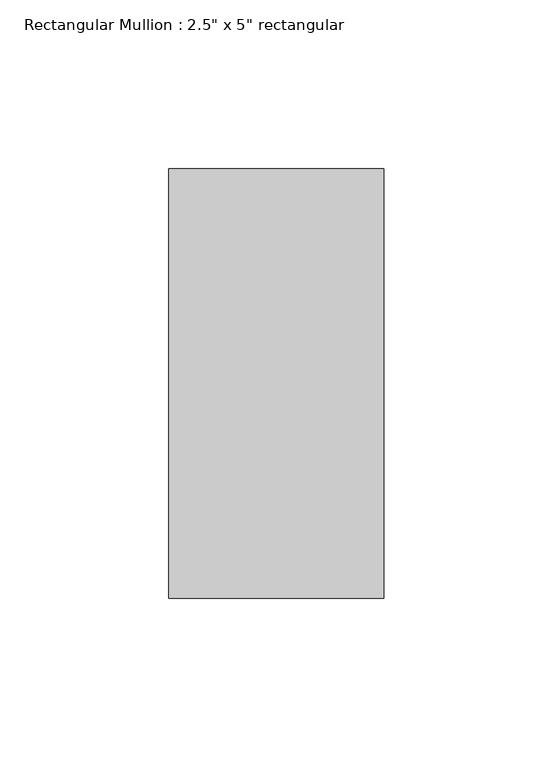
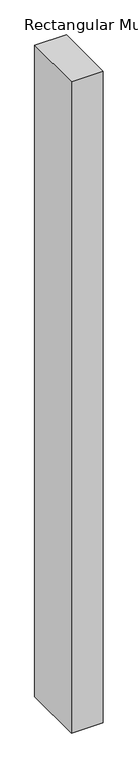
"""IFC4 building model written with IfcOpenShell, lengths in millimetres: member geometry."""

from ifc_helpers import new_model, si_unit, frame, origin, place, context, project, spatial, polyline, outline, extrude, source, transform, mapped, element, save


def member_2b4cd6f1(model_context):
    return source(origin(), model_context, "Body", "SweptSolid", [
        extrude(outline(polyline([(0.0, 63.5), (0.0, -63.5), (-63.5, -63.5), (-63.5, 63.5), (0.0, 63.5)])), frame((0.0, 0.0, -1377.9500001), z_axis=(0.0, 0.0, 1.0), x_axis=(1.0, 0.0, 0.0)), (0.0, 0.0, 1.0), 1377.9500001),
    ])


if __name__ == "__main__":
    model = new_model("IFC4")
    model_context = context("Model", 3, world=origin())
    ifc_project = project(units=[si_unit("LENGTHUNIT", "METRE", prefix="MILLI")], contexts=[model_context])
    site = spatial("IfcSite", under=ifc_project)
    building = spatial("IfcBuilding", under=site)
    placement = place(None, origin())
    member_shape = member_2b4cd6f1(model_context)
    element("IfcMember", 1, ObjectType="Rectangular Mullion : 2.5\" x 5\" rectangular", at=placement, inside=building, context=model_context, shape_type="MappedRepresentation", body=[
        mapped(member_shape, transform((0.0, 0.0, 0.0), x_axis=(1.0, 0.0, 0.0), y_axis=(0.0, 1.0, 0.0), z_axis=(0.0, 0.0, 1.0))),
    ])
    save(model, "model.ifc")

# Revit data of these elements
# Type "Rectangular Mullion : 2.5\" x 5\" rectangular"
#   built-in parameter 1007304 = 0.416667 (stored number, unit not read)
#   built-in parameter 1007301 = 0.104167 (stored number, unit not read)
#   built-in parameter 1007300 = 0.104167 (stored number, unit not read)
# Element 1 (IfcMember, "Rectangular Mullion : 2.5\" x 5\" rectangular")
#   Materials on its faces: "WINDOW FRAMING"
# Materials
#   "WINDOW FRAMING": class "Generic", colour RGB 120 120 120, transparency 0, Cost = 0
